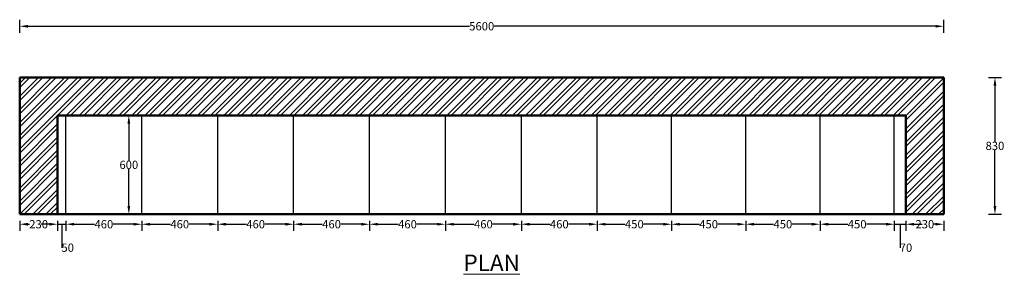
# Model space of a CAD drawing. Units: millimetres. Extents: x -472 to 16192, y -4730 to 4331.
# Tile 3 of 8: x 0 to 5967, y 2788 to 4331. Entities that reach past the tile are written whole.
import ezdxf

# ---------------------------------------------------------------- set-up
doc = ezdxf.new("R2010")
doc.units = ezdxf.units.MM
doc.header["$MEASUREMENT"] = 0
for name, color, linetype, lineweight in [('A-ANNO-DIMS', 2, 'Continuous', 18), ('A-ANNO-TEXT', 6, 'Continuous', 18), ('A-FURN', 8, 'Continuous', 25), ('A-WALL', 7, 'Continuous', 50), ('A-WALL-PATT', 8, 'Continuous', 13)]:
    doc.layers.add(name, color=color, linetype=linetype, lineweight=lineweight)
doc.styles.get("Standard").update_dxf_attribs({"font": 'arial.ttf'})
doc.dimstyles.get("Standard").update_dxf_attribs({"dimtxt": 50, "dimasz": 50, "dimexe": 40, "dimexo": 40, "dimgap": 0.09, "dimtad": 0, "dimtih": 1, "dimtoh": 1, "dimdec": 0, "dimzin": 0, "dimdsep": 46, "dimtxsty": 'Standard', "dimcen": 0.09, "dimclrd": 1, "dimclre": 3, "dimclrt": 6, "dimadec": 0, "dimazin": 0, "dimtfac": 1, "dimtdec": 0, "dimtofl": 0, "dimtmove": 0, "dimatfit": 3, "dimfxl": 40, "dimfxlon": 1, "dimtolj": 1, "dimtzin": 0, "dimarcsym": 0})

# ---------------------------------------------------------------- blocks, each defined once
blk = doc.blocks.new('*D1')
at = {"layer": 'A-ANNO-DIMS', "color": 0, "lineweight": -2, "transparency": 16777216}
for p, q in [((700, 3751.2), (621.3, 3751.2)), ((661.3, 3701.2), (661.3, 3476.8)), ((661.3, 3201.2), (661.3, 3425.6)), ((700, 3151.2), (621.3, 3151.2))]:
    blk.add_line(p, q, dxfattribs=at)
at = {"layer": 'A-ANNO-DIMS', "color": 0, "transparency": 16777216}
for points in [[(653, 3701.2), (669.6, 3701.2), (661.3, 3751.2)], [(653, 3201.2), (669.6, 3201.2), (661.3, 3151.2)]]:
    blk.add_solid(points, dxfattribs=at)
at = {"layer": 'Defpoints', "color": 0, "transparency": 16777216}
for p in [(740, 3751.2), (661.3, 3151.2), (740, 3151.2)]:
    blk.add_point(p, dxfattribs=at)
at = {"layer": 'A-ANNO-DIMS', "color": 0, "transparency": 16777216, "insert": (661.3, 3451.2), "char_height": 50, "attachment_point": 5}
blk.add_mtext('\\A1;600', dxfattribs=at)
blk = doc.blocks.new('*D2')
at = {"layer": 'A-ANNO-DIMS', "color": 0, "lineweight": -2, "transparency": 16777216}
for p, q in [((0, 3111.2), (0, 3051.2)), ((230, 3111.2), (230, 3051.2)), ((50, 3091.2), (59.3, 3091.2)), ((180, 3091.2), (170.7, 3091.2))]:
    blk.add_line(p, q, dxfattribs=at)
at = {"layer": 'A-ANNO-DIMS', "color": 0, "transparency": 16777216}
for points in [[(50, 3099.5), (50, 3082.9), (0, 3091.2)], [(180, 3099.5), (180, 3082.9), (230, 3091.2)]]:
    blk.add_solid(points, dxfattribs=at)
at = {"layer": 'Defpoints', "color": 0, "transparency": 16777216}
for p in [(0, 3151.2), (230, 3151.2), (230, 3091.2)]:
    blk.add_point(p, dxfattribs=at)
at = {"layer": 'A-ANNO-DIMS', "color": 0, "transparency": 16777216, "insert": (115, 3091.2), "char_height": 50, "attachment_point": 5}
blk.add_mtext('\\A1;230', dxfattribs=at)
blk = doc.blocks.new('*D3')
at = {"layer": 'A-ANNO-DIMS', "color": 0, "lineweight": -2, "transparency": 16777216}
for p, q in [((230, 3111.2), (230, 3051.2)), ((280, 3111.2), (280, 3051.2)), ((180, 3091.2), (130, 3091.2)), ((230, 3091.2), (280, 3091.2)), ((255, 3091.2), (255, 2949)), ((330, 3091.2), (380, 3091.2)), ((255, 2949), (255.2, 2949))]:
    blk.add_line(p, q, dxfattribs=at)
at = {"layer": 'A-ANNO-DIMS', "color": 0, "transparency": 16777216}
for points in [[(180, 3099.5), (180, 3082.9), (230, 3091.2)], [(330, 3099.5), (330, 3082.9), (280, 3091.2)]]:
    blk.add_solid(points, dxfattribs=at)
at = {"layer": 'Defpoints', "color": 0, "transparency": 16777216}
for p in [(230, 3151.2), (280, 3151.2), (280, 3091.2)]:
    blk.add_point(p, dxfattribs=at)
at = {"layer": 'A-ANNO-DIMS', "color": 0, "transparency": 16777216, "insert": (291, 2949), "char_height": 50, "attachment_point": 5}
blk.add_mtext('\\A1;50', dxfattribs=at)
blk = doc.blocks.new('*D4')
at = {"layer": 'A-ANNO-DIMS', "color": 0, "lineweight": -2, "transparency": 16777216}
for p, q in [((280, 3111.2), (280, 3051.2)), ((740, 3111.2), (740, 3051.2)), ((330, 3091.2), (453.8, 3091.2)), ((690, 3091.2), (566.2, 3091.2))]:
    blk.add_line(p, q, dxfattribs=at)
at = {"layer": 'A-ANNO-DIMS', "color": 0, "transparency": 16777216}
for points in [[(330, 3099.5), (330, 3082.9), (280, 3091.2)], [(690, 3099.5), (690, 3082.9), (740, 3091.2)]]:
    blk.add_solid(points, dxfattribs=at)
at = {"layer": 'Defpoints', "color": 0, "transparency": 16777216}
for p in [(280, 3151.2), (740, 3151.2), (740, 3091.2)]:
    blk.add_point(p, dxfattribs=at)
at = {"layer": 'A-ANNO-DIMS', "color": 0, "transparency": 16777216, "insert": (510, 3091.2), "char_height": 50, "attachment_point": 5}
blk.add_mtext('\\A1;460', dxfattribs=at)
blk = doc.blocks.new('*D5')
at = {"layer": 'A-ANNO-DIMS', "color": 0, "lineweight": -2, "transparency": 16777216}
for p, q in [((740, 3111.2), (740, 3051.2)), ((1200, 3111.2), (1200, 3051.2)), ((790, 3091.2), (913.8, 3091.2)), ((1150, 3091.2), (1026.2, 3091.2))]:
    blk.add_line(p, q, dxfattribs=at)
at = {"layer": 'A-ANNO-DIMS', "color": 0, "transparency": 16777216}
for points in [[(790, 3099.5), (790, 3082.9), (740, 3091.2)], [(1150, 3099.5), (1150, 3082.9), (1200, 3091.2)]]:
    blk.add_solid(points, dxfattribs=at)
at = {"layer": 'Defpoints', "color": 0, "transparency": 16777216}
for p in [(740, 3151.2), (1200, 3151.2), (1200, 3091.2)]:
    blk.add_point(p, dxfattribs=at)
at = {"layer": 'A-ANNO-DIMS', "color": 0, "transparency": 16777216, "insert": (970, 3091.2), "char_height": 50, "attachment_point": 5}
blk.add_mtext('\\A1;460', dxfattribs=at)
blk = doc.blocks.new('*D6')
at = {"layer": 'A-ANNO-DIMS', "color": 0, "lineweight": -2, "transparency": 16777216}
for p, q in [((1200, 3111.2), (1200, 3051.2)), ((1660, 3111.2), (1660, 3051.2)), ((1250, 3091.2), (1373.8, 3091.2)), ((1610, 3091.2), (1486.2, 3091.2))]:
    blk.add_line(p, q, dxfattribs=at)
at = {"layer": 'A-ANNO-DIMS', "color": 0, "transparency": 16777216}
for points in [[(1250, 3099.5), (1250, 3082.9), (1200, 3091.2)], [(1610, 3099.5), (1610, 3082.9), (1660, 3091.2)]]:
    blk.add_solid(points, dxfattribs=at)
at = {"layer": 'Defpoints', "color": 0, "transparency": 16777216}
for p in [(1200, 3151.2), (1660, 3151.2), (1660, 3091.2)]:
    blk.add_point(p, dxfattribs=at)
at = {"layer": 'A-ANNO-DIMS', "color": 0, "transparency": 16777216, "insert": (1430, 3091.2), "char_height": 50, "attachment_point": 5}
blk.add_mtext('\\A1;460', dxfattribs=at)
blk = doc.blocks.new('*D7')
at = {"layer": 'A-ANNO-DIMS', "color": 0, "lineweight": -2, "transparency": 16777216}
for p, q in [((1660, 3111.2), (1660, 3051.2)), ((2120, 3111.2), (2120, 3051.2)), ((1710, 3091.2), (1833.8, 3091.2)), ((2070, 3091.2), (1946.2, 3091.2))]:
    blk.add_line(p, q, dxfattribs=at)
at = {"layer": 'A-ANNO-DIMS', "color": 0, "transparency": 16777216}
for points in [[(1710, 3099.5), (1710, 3082.9), (1660, 3091.2)], [(2070, 3099.5), (2070, 3082.9), (2120, 3091.2)]]:
    blk.add_solid(points, dxfattribs=at)
at = {"layer": 'Defpoints', "color": 0, "transparency": 16777216}
for p in [(1660, 3151.2), (2120, 3151.2), (2120, 3091.2)]:
    blk.add_point(p, dxfattribs=at)
at = {"layer": 'A-ANNO-DIMS', "color": 0, "transparency": 16777216, "insert": (1890, 3091.2), "char_height": 50, "attachment_point": 5}
blk.add_mtext('\\A1;460', dxfattribs=at)
blk = doc.blocks.new('*D8')
at = {"layer": 'A-ANNO-DIMS', "color": 0, "lineweight": -2, "transparency": 16777216}
for p, q in [((2120, 3111.2), (2120, 3051.2)), ((2580, 3111.2), (2580, 3051.2)), ((2170, 3091.2), (2293.8, 3091.2)), ((2530, 3091.2), (2406.2, 3091.2))]:
    blk.add_line(p, q, dxfattribs=at)
at = {"layer": 'A-ANNO-DIMS', "color": 0, "transparency": 16777216}
for points in [[(2170, 3099.5), (2170, 3082.9), (2120, 3091.2)], [(2530, 3099.5), (2530, 3082.9), (2580, 3091.2)]]:
    blk.add_solid(points, dxfattribs=at)
at = {"layer": 'Defpoints', "color": 0, "transparency": 16777216}
for p in [(2120, 3151.2), (2580, 3151.2), (2580, 3091.2)]:
    blk.add_point(p, dxfattribs=at)
at = {"layer": 'A-ANNO-DIMS', "color": 0, "transparency": 16777216, "insert": (2350, 3091.2), "char_height": 50, "attachment_point": 5}
blk.add_mtext('\\A1;460', dxfattribs=at)
blk = doc.blocks.new('*D9')
at = {"layer": 'A-ANNO-DIMS', "color": 0, "lineweight": -2, "transparency": 16777216}
for p, q in [((2580, 3111.2), (2580, 3051.2)), ((3040, 3111.2), (3040, 3051.2)), ((2630, 3091.2), (2753.8, 3091.2)), ((2990, 3091.2), (2866.2, 3091.2))]:
    blk.add_line(p, q, dxfattribs=at)
at = {"layer": 'A-ANNO-DIMS', "color": 0, "transparency": 16777216}
for points in [[(2630, 3099.5), (2630, 3082.9), (2580, 3091.2)], [(2990, 3099.5), (2990, 3082.9), (3040, 3091.2)]]:
    blk.add_solid(points, dxfattribs=at)
at = {"layer": 'Defpoints', "color": 0, "transparency": 16777216}
for p in [(2580, 3151.2), (3040, 3151.2), (3040, 3091.2)]:
    blk.add_point(p, dxfattribs=at)
at = {"layer": 'A-ANNO-DIMS', "color": 0, "transparency": 16777216, "insert": (2810, 3091.2), "char_height": 50, "attachment_point": 5}
blk.add_mtext('\\A1;460', dxfattribs=at)
blk = doc.blocks.new('*D10')
at = {"layer": 'A-ANNO-DIMS', "color": 0, "lineweight": -2, "transparency": 16777216}
for p, q in [((3040, 3111.2), (3040, 3051.2)), ((3500, 3111.2), (3500, 3051.2)), ((3090, 3091.2), (3213.8, 3091.2)), ((3450, 3091.2), (3326.2, 3091.2))]:
    blk.add_line(p, q, dxfattribs=at)
at = {"layer": 'A-ANNO-DIMS', "color": 0, "transparency": 16777216}
for points in [[(3090, 3099.5), (3090, 3082.9), (3040, 3091.2)], [(3450, 3099.5), (3450, 3082.9), (3500, 3091.2)]]:
    blk.add_solid(points, dxfattribs=at)
at = {"layer": 'Defpoints', "color": 0, "transparency": 16777216}
for p in [(3040, 3151.2), (3500, 3151.2), (3500, 3091.2)]:
    blk.add_point(p, dxfattribs=at)
at = {"layer": 'A-ANNO-DIMS', "color": 0, "transparency": 16777216, "insert": (3270, 3091.2), "char_height": 50, "attachment_point": 5}
blk.add_mtext('\\A1;460', dxfattribs=at)
blk = doc.blocks.new('*D11')
at = {"layer": 'A-ANNO-DIMS', "color": 0, "lineweight": -2, "transparency": 16777216}
for p, q in [((3500, 3111.2), (3500, 3051.2)), ((3950, 3111.2), (3950, 3051.2)), ((3550, 3091.2), (3668.8, 3091.2)), ((3900, 3091.2), (3781.2, 3091.2))]:
    blk.add_line(p, q, dxfattribs=at)
at = {"layer": 'A-ANNO-DIMS', "color": 0, "transparency": 16777216}
for points in [[(3550, 3099.5), (3550, 3082.9), (3500, 3091.2)], [(3900, 3099.5), (3900, 3082.9), (3950, 3091.2)]]:
    blk.add_solid(points, dxfattribs=at)
at = {"layer": 'Defpoints', "color": 0, "transparency": 16777216}
for p in [(3500, 3151.2), (3950, 3151.2), (3950, 3091.2)]:
    blk.add_point(p, dxfattribs=at)
at = {"layer": 'A-ANNO-DIMS', "color": 0, "transparency": 16777216, "insert": (3725, 3091.2), "char_height": 50, "attachment_point": 5}
blk.add_mtext('\\A1;450', dxfattribs=at)
blk = doc.blocks.new('*D12')
at = {"layer": 'A-ANNO-DIMS', "color": 0, "lineweight": -2, "transparency": 16777216}
for p, q in [((3950, 3111.2), (3950, 3051.2)), ((4400, 3111.2), (4400, 3051.2)), ((4000, 3091.2), (4118.8, 3091.2)), ((4350, 3091.2), (4231.2, 3091.2))]:
    blk.add_line(p, q, dxfattribs=at)
at = {"layer": 'A-ANNO-DIMS', "color": 0, "transparency": 16777216}
for points in [[(4000, 3099.5), (4000, 3082.9), (3950, 3091.2)], [(4350, 3099.5), (4350, 3082.9), (4400, 3091.2)]]:
    blk.add_solid(points, dxfattribs=at)
at = {"layer": 'Defpoints', "color": 0, "transparency": 16777216}
for p in [(3950, 3151.2), (4400, 3151.2), (4400, 3091.2)]:
    blk.add_point(p, dxfattribs=at)
at = {"layer": 'A-ANNO-DIMS', "color": 0, "transparency": 16777216, "insert": (4175, 3091.2), "char_height": 50, "attachment_point": 5}
blk.add_mtext('\\A1;450', dxfattribs=at)
blk = doc.blocks.new('*D13')
at = {"layer": 'A-ANNO-DIMS', "color": 0, "lineweight": -2, "transparency": 16777216}
for p, q in [((4400, 3111.2), (4400, 3051.2)), ((4850, 3111.2), (4850, 3051.2)), ((4450, 3091.2), (4568.8, 3091.2)), ((4800, 3091.2), (4681.2, 3091.2))]:
    blk.add_line(p, q, dxfattribs=at)
at = {"layer": 'A-ANNO-DIMS', "color": 0, "transparency": 16777216}
for points in [[(4450, 3099.5), (4450, 3082.9), (4400, 3091.2)], [(4800, 3099.5), (4800, 3082.9), (4850, 3091.2)]]:
    blk.add_solid(points, dxfattribs=at)
at = {"layer": 'Defpoints', "color": 0, "transparency": 16777216}
for p in [(4400, 3151.2), (4850, 3151.2), (4850, 3091.2)]:
    blk.add_point(p, dxfattribs=at)
at = {"layer": 'A-ANNO-DIMS', "color": 0, "transparency": 16777216, "insert": (4625, 3091.2), "char_height": 50, "attachment_point": 5}
blk.add_mtext('\\A1;450', dxfattribs=at)
blk = doc.blocks.new('*D14')
at = {"layer": 'A-ANNO-DIMS', "color": 0, "lineweight": -2, "transparency": 16777216}
for p, q in [((4850, 3111.2), (4850, 3051.2)), ((5300, 3111.2), (5300, 3051.2)), ((4900, 3091.2), (5018.8, 3091.2)), ((5250, 3091.2), (5131.2, 3091.2))]:
    blk.add_line(p, q, dxfattribs=at)
at = {"layer": 'A-ANNO-DIMS', "color": 0, "transparency": 16777216}
for points in [[(4900, 3099.5), (4900, 3082.9), (4850, 3091.2)], [(5250, 3099.5), (5250, 3082.9), (5300, 3091.2)]]:
    blk.add_solid(points, dxfattribs=at)
at = {"layer": 'Defpoints', "color": 0, "transparency": 16777216}
for p in [(4850, 3151.2), (5300, 3151.2), (5300, 3091.2)]:
    blk.add_point(p, dxfattribs=at)
at = {"layer": 'A-ANNO-DIMS', "color": 0, "transparency": 16777216, "insert": (5075, 3091.2), "char_height": 50, "attachment_point": 5}
blk.add_mtext('\\A1;450', dxfattribs=at)
blk = doc.blocks.new('*D15')
at = {"layer": 'A-ANNO-DIMS', "color": 0, "lineweight": -2, "transparency": 16777216}
for p, q in [((5300, 3111.2), (5300, 3051.2)), ((5370, 3111.2), (5370, 3051.2)), ((5250, 3091.2), (5200, 3091.2)), ((5300, 3091.2), (5370, 3091.2)), ((5335, 3091.2), (5335, 2949)), ((5420, 3091.2), (5470, 3091.2)), ((5335, 2949), (5335.2, 2949))]:
    blk.add_line(p, q, dxfattribs=at)
at = {"layer": 'A-ANNO-DIMS', "color": 0, "transparency": 16777216}
for points in [[(5250, 3099.5), (5250, 3082.9), (5300, 3091.2)], [(5420, 3099.5), (5420, 3082.9), (5370, 3091.2)]]:
    blk.add_solid(points, dxfattribs=at)
at = {"layer": 'Defpoints', "color": 0, "transparency": 16777216}
for p in [(5300, 3151.2), (5370, 3151.2), (5370, 3091.2)]:
    blk.add_point(p, dxfattribs=at)
at = {"layer": 'A-ANNO-DIMS', "color": 0, "transparency": 16777216, "insert": (5370.8, 2949), "char_height": 50, "attachment_point": 5}
blk.add_mtext('\\A1;70', dxfattribs=at)
blk = doc.blocks.new('*D16')
at = {"layer": 'A-ANNO-DIMS', "color": 0, "lineweight": -2, "transparency": 16777216}
for p, q in [((5370, 3111.2), (5370, 3051.2)), ((5600, 3111.2), (5600, 3051.2)), ((5420, 3091.2), (5429.3, 3091.2)), ((5550, 3091.2), (5540.7, 3091.2))]:
    blk.add_line(p, q, dxfattribs=at)
at = {"layer": 'A-ANNO-DIMS', "color": 0, "transparency": 16777216}
for points in [[(5420, 3099.5), (5420, 3082.9), (5370, 3091.2)], [(5550, 3099.5), (5550, 3082.9), (5600, 3091.2)]]:
    blk.add_solid(points, dxfattribs=at)
at = {"layer": 'Defpoints', "color": 0, "transparency": 16777216}
for p in [(5370, 3151.2), (5600, 3151.2), (5600, 3091.2)]:
    blk.add_point(p, dxfattribs=at)
at = {"layer": 'A-ANNO-DIMS', "color": 0, "transparency": 16777216, "insert": (5485, 3091.2), "char_height": 50, "attachment_point": 5}
blk.add_mtext('\\A1;230', dxfattribs=at)
blk = doc.blocks.new('*D95')
at = {"layer": 'A-ANNO-DIMS', "color": 3, "lineweight": -2, "transparency": 16777216}
for p, q in [((0, 4251.2), (0, 4331.2)), ((5600, 4251.2), (5600, 4331.2))]:
    blk.add_line(p, q, dxfattribs=at)
at = {"layer": 'A-ANNO-DIMS', "color": 1, "lineweight": -2, "transparency": 16777216}
for p, q in [((50, 4291.2), (2725.3, 4291.2)), ((5550, 4291.2), (2874.7, 4291.2))]:
    blk.add_line(p, q, dxfattribs=at)
at = {"layer": 'A-ANNO-DIMS', "color": 1, "transparency": 16777216}
for points in [[(50, 4299.5), (50, 4282.9), (0, 4291.2)], [(5550, 4299.5), (5550, 4282.9), (5600, 4291.2)]]:
    blk.add_solid(points, dxfattribs=at)
at = {"layer": 'Defpoints', "color": 0, "transparency": 16777216}
for p in [(5600, 4291.2), (0, 3981.2), (5600, 3981.2)]:
    blk.add_point(p, dxfattribs=at)
at = {"layer": 'A-ANNO-DIMS', "color": 6, "transparency": 16777216, "insert": (2800, 4291.2), "char_height": 50, "attachment_point": 5}
blk.add_mtext('\\A1;5600', dxfattribs=at)
blk = doc.blocks.new('*D96')
at = {"layer": 'A-ANNO-DIMS', "color": 3, "lineweight": -2, "transparency": 16777216}
for p, q in [((5870, 3981.2), (5950, 3981.2)), ((5870, 3151.2), (5950, 3151.2))]:
    blk.add_line(p, q, dxfattribs=at)
at = {"layer": 'A-ANNO-DIMS', "color": 1, "lineweight": -2, "transparency": 16777216}
for p, q in [((5910, 3931.2), (5910, 3591.8)), ((5910, 3201.2), (5910, 3540.6))]:
    blk.add_line(p, q, dxfattribs=at)
at = {"layer": 'A-ANNO-DIMS', "color": 1, "transparency": 16777216}
for points in [[(5901.7, 3931.2), (5918.3, 3931.2), (5910, 3981.2)], [(5901.7, 3201.2), (5918.3, 3201.2), (5910, 3151.2)]]:
    blk.add_solid(points, dxfattribs=at)
at = {"layer": 'Defpoints', "color": 0, "transparency": 16777216}
for p in [(5600, 3981.2), (5600, 3151.2), (5910, 3151.2)]:
    blk.add_point(p, dxfattribs=at)
at = {"layer": 'A-ANNO-DIMS', "color": 6, "transparency": 16777216, "insert": (5910, 3566.2), "char_height": 50, "attachment_point": 5}
blk.add_mtext('\\A1;830', dxfattribs=at)

msp = doc.modelspace()

# ---------------------------------------------------------------- hatches: boundary and pattern name
at = {"layer": 'A-WALL-PATT'}
h = msp.add_hatch(dxfattribs=at)
h.set_pattern_fill('ANSI32', color=256, scale=150)
h.set_pattern_definition([(45, (0, 3151.193), (-39.77476, 39.77476), []), (45, (26.517, 3151.193), (-39.77476, 39.77476), [])])
h.paths.add_polyline_path([(5370, 3751.2), (5370, 3151.2), (5600, 3151.2), (5600, 3981.2), (0, 3981.2), (0, 3151.2), (230, 3151.2), (230, 3751.2)])

# ---------------------------------------------------------------- linework, layer by layer
at = {"layer": 'A-FURN'}
for p, q in [((280, 3151.2), (280, 3751.2)), ((740, 3151.2), (740, 3751.2)), ((1200, 3151.2), (1200, 3751.2)), ((1660, 3151.2), (1660, 3751.2)), ((2120, 3151.2), (2120, 3751.2)), ((2580, 3151.2), (2580, 3751.2)), ((3040, 3151.2), (3040, 3751.2)), ((3500, 3151.2), (3500, 3751.2)), ((3950, 3151.2), (3950, 3751.2)), ((4400, 3151.2), (4400, 3751.2)), ((4850, 3151.2), (4850, 3751.2)), ((5300, 3151.2), (5300, 3751.2))]:
    msp.add_line(p, q, dxfattribs=at)
at = {"layer": 'A-WALL'}
for p, q in [((0, 3151.2), (0, 3981.2)), ((0, 3981.2), (5600, 3981.2)), ((5600, 3151.2), (5600, 3981.2)), ((230, 3151.2), (230, 3751.2)), ((230, 3751.2), (5370, 3751.2)), ((5370, 3151.2), (5370, 3751.2)), ((0, 3151.2), (5600, 3151.2))]:
    msp.add_line(p, q, dxfattribs=at)

# ---------------------------------------------------------------- texts
at = {"layer": 'A-ANNO-TEXT', "insert": (2689.3, 2907.6), "char_height": 100, "attachment_point": 1}
msp.add_mtext_dynamic_manual_height_columns('{\\fArial|b1|i0|c0|p34;\\LPLAN}', width=3435.915, gutter_width=1, heights=[0], dxfattribs=at)

# ---------------------------------------------------------------- dimensions: what is measured, and where the dimension line sits
at = {"layer": 'A-ANNO-DIMS'}
for base, p1, p2, override, picture, middle in [((5600, 4291.2), (0, 3981.2), (5600, 3981.2), {"dimdec": 0, "dimlfac": 1, "dimrnd": 0, "dimzin": 0, "dimdsep": 46, "dimlunit": 2}, '*D95', (2800, 4291.2)), ((230, 3091.2), (0, 3151.2), (230, 3151.2), {"dimclrd": 0, "dimclre": 0, "dimclrt": 0}, '*D2', (115, 3091.2)), ((280, 3091.2), (230, 3151.2), (280, 3151.2), {"dimclrd": 0, "dimclre": 0, "dimclrt": 0, "dimtmove": 1}, '*D3', (255.3, 2949)), ((740, 3091.2), (280, 3151.2), (740, 3151.2), {"dimclrd": 0, "dimclre": 0, "dimclrt": 0, "dimtmove": 1}, '*D4', (510, 3091.2)), ((1200, 3091.2), (740, 3151.2), (1200, 3151.2), {"dimclrd": 0, "dimclre": 0, "dimclrt": 0, "dimtmove": 1}, '*D5', (970, 3091.2)), ((1660, 3091.2), (1200, 3151.2), (1660, 3151.2), {"dimclrd": 0, "dimclre": 0, "dimclrt": 0, "dimtmove": 1}, '*D6', (1430, 3091.2)), ((2120, 3091.2), (1660, 3151.2), (2120, 3151.2), {"dimclrd": 0, "dimclre": 0, "dimclrt": 0, "dimtmove": 1}, '*D7', (1890, 3091.2)), ((2580, 3091.2), (2120, 3151.2), (2580, 3151.2), {"dimclrd": 0, "dimclre": 0, "dimclrt": 0, "dimtmove": 1}, '*D8', (2350, 3091.2)), ((3040, 3091.2), (2580, 3151.2), (3040, 3151.2), {"dimclrd": 0, "dimclre": 0, "dimclrt": 0, "dimtmove": 1}, '*D9', (2810, 3091.2)), ((3500, 3091.2), (3040, 3151.2), (3500, 3151.2), {"dimclrd": 0, "dimclre": 0, "dimclrt": 0, "dimtmove": 1}, '*D10', (3270, 3091.2)), ((3950, 3091.2), (3500, 3151.2), (3950, 3151.2), {"dimclrd": 0, "dimclre": 0, "dimclrt": 0, "dimtmove": 1}, '*D11', (3725, 3091.2)), ((4400, 3091.2), (3950, 3151.2), (4400, 3151.2), {"dimclrd": 0, "dimclre": 0, "dimclrt": 0, "dimtmove": 1}, '*D12', (4175, 3091.2)), ((4850, 3091.2), (4400, 3151.2), (4850, 3151.2), {"dimclrd": 0, "dimclre": 0, "dimclrt": 0, "dimtmove": 1}, '*D13', (4625, 3091.2)), ((5300, 3091.2), (4850, 3151.2), (5300, 3151.2), {"dimclrd": 0, "dimclre": 0, "dimclrt": 0, "dimtmove": 1}, '*D14', (5075, 3091.2)), ((5370, 3091.2), (5300, 3151.2), (5370, 3151.2), {"dimclrd": 0, "dimclre": 0, "dimclrt": 0, "dimtmove": 1}, '*D15', (5335.3, 2949)), ((5600, 3091.2), (5370, 3151.2), (5600, 3151.2), {"dimclrd": 0, "dimclre": 0, "dimclrt": 0, "dimtmove": 1}, '*D16', (5485, 3091.2))]:
    dim = msp.add_linear_dim(base=base, p1=p1, p2=p2, dimstyle='Standard', override=override, dxfattribs=at)
    dim.commit()
    dim.dimension.update_dxf_attribs({"geometry": picture, "text_midpoint": middle})
for base, p1, p2, override, picture, middle in [((5910, 3151.2), (5600, 3981.2), (5600, 3151.2), {"dimdec": 0, "dimlfac": 1, "dimrnd": 0, "dimzin": 0, "dimdsep": 46, "dimlunit": 2}, '*D96', (5910, 3566.2)), ((661.3, 3151.2), (740, 3751.2), (740, 3151.2), {"dimclrd": 0, "dimclre": 0, "dimclrt": 0}, '*D1', (661.3, 3451.2))]:
    dim = msp.add_linear_dim(base=base, p1=p1, p2=p2, angle=90, dimstyle='Standard', override=override, dxfattribs=at)
    dim.commit()
    dim.dimension.update_dxf_attribs({"geometry": picture, "text_midpoint": middle})

doc.saveas('drawing.dxf')
